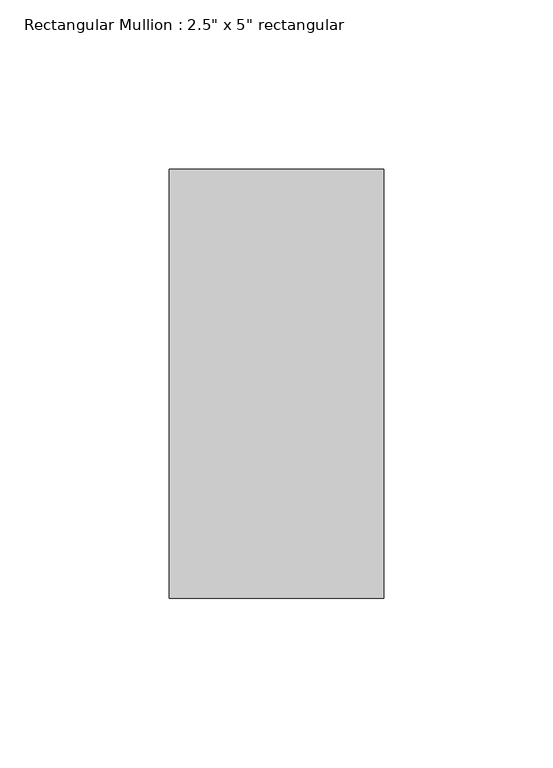
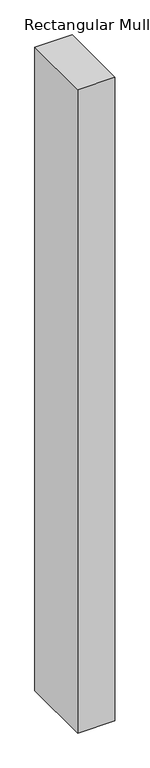
"""IFC4 building model written with IfcOpenShell, lengths in millimetres: member geometry."""

from ifc_helpers import new_model, si_unit, frame, origin, place, context, project, spatial, polyline, outline, extrude, source, transform, mapped, element, save


def member_ffab42ea(model_context):
    return source(origin(), model_context, "Body", "SweptSolid", [
        extrude(outline(polyline([(31.75, 63.5), (31.75, -63.5), (-31.75, -63.5), (-31.75, 63.5), (31.75, 63.5)])), frame((0.0, 0.0, -1164.1666667), z_axis=(0.0, 0.0, 1.0), x_axis=(1.0, 0.0, 0.0)), (0.0, 0.0, 1.0), 1164.1666667),
    ])


if __name__ == "__main__":
    model = new_model("IFC4")
    model_context = context("Model", 3, world=origin())
    ifc_project = project(units=[si_unit("LENGTHUNIT", "METRE", prefix="MILLI")], contexts=[model_context])
    site = spatial("IfcSite", under=ifc_project)
    building = spatial("IfcBuilding", under=site)
    placement = place(None, origin())
    member_shape = member_ffab42ea(model_context)
    element("IfcMember", 1, ObjectType="Rectangular Mullion : 2.5\" x 5\" rectangular", at=placement, inside=building, context=model_context, shape_type="MappedRepresentation", body=[
        mapped(member_shape, transform((0.0, 0.0, 0.0), x_axis=(1.0, 0.0, 0.0), y_axis=(0.0, 1.0, 0.0), z_axis=(0.0, 0.0, 1.0))),
    ])
    save(model, "model.ifc")

# Revit data of these elements
# Type "Rectangular Mullion : 2.5\" x 5\" rectangular"
#   built-in parameter 1007304 = 0.416667 (stored number, unit not read)
#   built-in parameter 1007301 = 0.104167 (stored number, unit not read)
#   built-in parameter 1007300 = 0.104167 (stored number, unit not read)
# Element 1 (IfcMember, "Rectangular Mullion : 2.5\" x 5\" rectangular")
#   Materials on its faces: "Aluminum"
# Materials
#   "Aluminum": class "Metal", colour RGB 247 247 247, transparency 0, Description = "Aluminum 6061", Cost = 0
